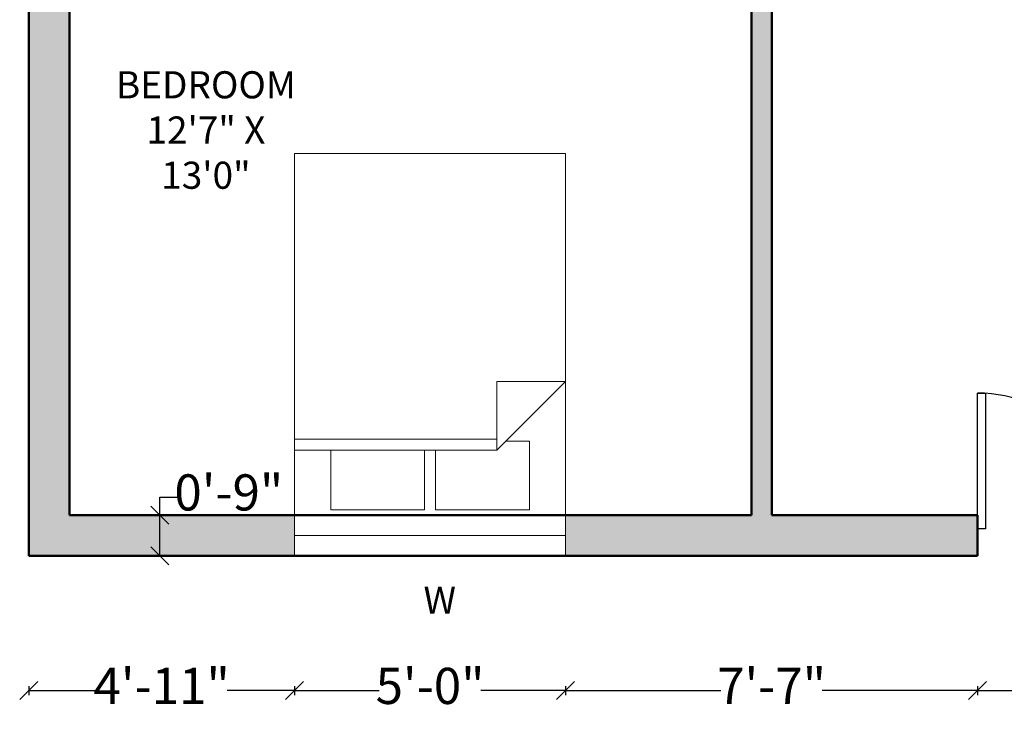
# Model space of a CAD drawing. Units: inches. Extents: x 2395 to 2921, y 528 to 1164.
# Tile 1 of 5: x 2444 to 2662, y 535 to 688. Entities that reach past the tile are written whole.
import ezdxf

# ---------------------------------------------------------------- set-up
doc = ezdxf.new("R2010")
doc.units = ezdxf.units.IN
for name, color, linetype, lineweight in [('A-ANNO-DIMS', 2, 'Continuous', 18), ('A-ANNO-TEXT', 7, 'Continuous', 18), ('A-AREA-IDEN', 7, 'Continuous', 25), ('A-DOOR', 3, 'Continuous', 25), ('A-FURN', 8, 'Continuous', 18), ('A-GLAZ', 4, 'Continuous', 18), ('A-WALL', 162, 'Continuous', 50), ('A-WALL-PATT', 162, 'Continuous', 13)]:
    doc.layers.add(name, color=color, linetype=linetype, lineweight=lineweight)
doc.styles.get("Standard").update_dxf_attribs({"font": 'arial.ttf'})
doc.dimstyles.new('ISO-25', dxfattribs={"dimtxt": 8, "dimasz": 4, "dimexe": 1, "dimexo": 1, "dimtad": 0, "dimtih": 1, "dimtoh": 1, "dimlunit": 3, "dimtxsty": 'Standard', "dimblk": 'OBLIQUE', "dimcen": 2.5, "dimadec": 0, "dimazin": 0, "dimtfac": 1, "dimtmove": 0, "dimatfit": 3, "dimfxl": 1, "dimfxlon": 1, "dimarcsym": 0})

# ---------------------------------------------------------------- blocks, each defined once
blk = doc.blocks.new('*U6')
for p, q in [((0, 0), (0, -6)), ((30, 0), (30, -6))]:
    blk.add_line(p, q)
blk.add_lwpolyline([(0, 0), (0, 30), (1.75, 30), (1.75, 0)], close=True)
blk.add_arc((0, 0), 30, 0, 90)
blk = doc.blocks.new('Bed - Queen')
for p, q in [((0, -80.00003), (0, 0)), ((0, 0), (59.99999, 0)), ((59.99999, 0), (59.99999, -80.00003)), ((7.99999, -1.2), (28.79998, -1.2)), ((7.99999, -14.4), (7.99999, -1.2)), ((28.79998, -1.2), (28.79998, -14.4)), ((31.19999, -1.2), (51.99999, -1.2)), ((31.19999, -14.4), (31.19999, -1.2)), ((51.99999, -1.2), (51.99999, -16.4)), ((0, -14.4), (44.8, -14.4)), ((59.99999, -29.6), (44.8, -14.4)), ((44.8, -14.4), (44.8, -29.6)), ((44.8, -16.8), (0, -16.8)), ((51.99999, -16.4), (46.79936, -16.4)), ((44.8, -29.6), (59.99999, -29.6)), ((59.99999, -80.00003), (0, -80.00003))]:
    blk.add_line(p, q)
blk = doc.blocks.new('_Oblique')
at = {"color": 0, "linetype": 'ByBlock', "lineweight": -2}
blk.add_line((-0.5, -0.5), (0.5, 0.5), dxfattribs=at)
blk = doc.blocks.new('*D42')
at = {"layer": 'A-ANNO-DIMS', "color": 0, "lineweight": -2, "transparency": 16777216}
for p, q in [((2446.2, 541.05), (2446.2, 539.05)), ((2505.03, 541.05), (2505.03, 539.05)), ((2446.2, 540.05), (2461.09, 540.05)), ((2505.03, 540.05), (2490.14, 540.05))]:
    blk.add_line(p, q, dxfattribs=at)
at = {"layer": 'Defpoints', "color": 0, "transparency": 16777216}
for p in [(2446.2, 569.85), (2505.03, 569.85), (2505.03, 540.05)]:
    blk.add_point(p, dxfattribs=at)
at = {"layer": 'A-ANNO-DIMS', "color": 0, "lineweight": -2, "transparency": 16777216, "xscale": 4, "yscale": 4, "zscale": 4, "rotation": 180}
blk.add_blockref('_Oblique', (2446.2, 540.05), dxfattribs=at)
at = {"layer": 'A-ANNO-DIMS', "color": 0, "lineweight": -2, "transparency": 16777216, "xscale": 4, "yscale": 4, "zscale": 4}
blk.add_blockref('_Oblique', (2505.03, 540.05), dxfattribs=at)
at = {"layer": 'A-ANNO-DIMS', "color": 0, "transparency": 16777216, "insert": (2475.62, 540.05), "char_height": 8, "attachment_point": 5}
blk.add_mtext('4\'-11"', dxfattribs=at)
blk = doc.blocks.new('*D43')
at = {"layer": 'A-ANNO-DIMS', "color": 0, "lineweight": -2, "transparency": 16777216}
for p, q in [((2505.03, 541.05), (2505.03, 539.05)), ((2565.03, 541.05), (2565.03, 539.05)), ((2505.03, 540.05), (2523.77, 540.05)), ((2565.03, 540.05), (2546.29, 540.05))]:
    blk.add_line(p, q, dxfattribs=at)
at = {"layer": 'Defpoints', "color": 0, "transparency": 16777216}
for p in [(2505.03, 569.85), (2565.03, 569.85), (2565.03, 540.05)]:
    blk.add_point(p, dxfattribs=at)
at = {"layer": 'A-ANNO-DIMS', "color": 0, "lineweight": -2, "transparency": 16777216, "xscale": 4, "yscale": 4, "zscale": 4, "rotation": 180}
blk.add_blockref('_Oblique', (2505.03, 540.05), dxfattribs=at)
at = {"layer": 'A-ANNO-DIMS', "color": 0, "lineweight": -2, "transparency": 16777216, "xscale": 4, "yscale": 4, "zscale": 4}
blk.add_blockref('_Oblique', (2565.03, 540.05), dxfattribs=at)
at = {"layer": 'A-ANNO-DIMS', "color": 0, "transparency": 16777216, "insert": (2535.03, 540.05), "char_height": 8, "attachment_point": 5}
blk.add_mtext('5\'-0"', dxfattribs=at)
blk = doc.blocks.new('*D44')
at = {"layer": 'A-ANNO-DIMS', "color": 0, "lineweight": -2, "transparency": 16777216}
for p, q in [((2565.03, 541.05), (2565.03, 539.05)), ((2656.2, 541.05), (2656.2, 539.05)), ((2565.03, 540.05), (2599.39, 540.05)), ((2656.2, 540.05), (2621.84, 540.05))]:
    blk.add_line(p, q, dxfattribs=at)
at = {"layer": 'Defpoints', "color": 0, "transparency": 16777216}
for p in [(2565.03, 569.85), (2656.2, 569.85), (2656.2, 540.05)]:
    blk.add_point(p, dxfattribs=at)
at = {"layer": 'A-ANNO-DIMS', "color": 0, "lineweight": -2, "transparency": 16777216, "xscale": 4, "yscale": 4, "zscale": 4, "rotation": 180}
blk.add_blockref('_Oblique', (2565.03, 540.05), dxfattribs=at)
at = {"layer": 'A-ANNO-DIMS', "color": 0, "lineweight": -2, "transparency": 16777216, "xscale": 4, "yscale": 4, "zscale": 4}
blk.add_blockref('_Oblique', (2656.2, 540.05), dxfattribs=at)
at = {"layer": 'A-ANNO-DIMS', "color": 0, "transparency": 16777216, "insert": (2610.62, 540.05), "char_height": 8, "attachment_point": 5}
blk.add_mtext('7\'-7"', dxfattribs=at)
blk = doc.blocks.new('*D45')
at = {"layer": 'A-ANNO-DIMS', "color": 0, "lineweight": -2, "transparency": 16777216}
for p, q in [((2656.2, 541.05), (2656.2, 539.05)), ((2716.2, 541.05), (2716.2, 539.05)), ((2656.2, 540.05), (2674.94, 540.05)), ((2716.2, 540.05), (2697.46, 540.05))]:
    blk.add_line(p, q, dxfattribs=at)
at = {"layer": 'Defpoints', "color": 0, "transparency": 16777216}
for p in [(2656.2, 569.85), (2716.2, 569.85), (2716.2, 540.05)]:
    blk.add_point(p, dxfattribs=at)
at = {"layer": 'A-ANNO-DIMS', "color": 0, "lineweight": -2, "transparency": 16777216, "xscale": 4, "yscale": 4, "zscale": 4, "rotation": 180}
blk.add_blockref('_Oblique', (2656.2, 540.05), dxfattribs=at)
at = {"layer": 'A-ANNO-DIMS', "color": 0, "lineweight": -2, "transparency": 16777216, "xscale": 4, "yscale": 4, "zscale": 4}
blk.add_blockref('_Oblique', (2716.2, 540.05), dxfattribs=at)
at = {"layer": 'A-ANNO-DIMS', "color": 0, "transparency": 16777216, "insert": (2686.2, 540.05), "char_height": 8, "attachment_point": 5}
blk.add_mtext('5\'-0"', dxfattribs=at)
blk = doc.blocks.new('*D50')
at = {"layer": 'A-ANNO-DIMS', "color": 0, "lineweight": -2, "transparency": 16777216}
for p, q in [((2475.23, 578.85), (2475.23, 582.85)), ((2475.23, 582.85), (2479.23, 582.85)), ((2476.23, 578.85), (2474.23, 578.85)), ((2475.23, 569.85), (2475.23, 578.85)), ((2476.23, 569.85), (2474.23, 569.85))]:
    blk.add_line(p, q, dxfattribs=at)
at = {"layer": 'Defpoints', "color": 0, "transparency": 16777216}
for p in [(2475.23, 578.85), (2505.03, 578.85), (2505.03, 569.85)]:
    blk.add_point(p, dxfattribs=at)
at = {"layer": 'A-ANNO-DIMS', "color": 0, "lineweight": -2, "transparency": 16777216, "xscale": 4, "yscale": 4, "zscale": 4}
for p, rotation in [((2475.23, 578.85), 90), ((2475.23, 569.85), 270)]:
    blk.add_blockref('_Oblique', p, dxfattribs=dict(at, rotation=rotation))
at = {"layer": 'A-ANNO-DIMS', "color": 0, "transparency": 16777216, "insert": (2490.49, 582.85), "char_height": 8, "attachment_point": 5}
blk.add_mtext('0\'-9"', dxfattribs=at)
blk = doc.blocks.new('*D51')
at = {"layer": 'A-ANNO-DIMS', "color": 0, "lineweight": -2, "transparency": 16777216}
for p, q in [((2606.2, 1150.65), (2606.2, 1152.65)), ((2606.2, 1151.65), (2610.7, 1151.65)), ((2610.7, 1150.65), (2610.7, 1152.65)), ((2610.7, 1151.65), (2614.7, 1151.65))]:
    blk.add_line(p, q, dxfattribs=at)
at = {"layer": 'Defpoints', "color": 0, "transparency": 16777216}
for p in [(2610.7, 1151.65), (2606.2, 578.85), (2610.7, 578.85)]:
    blk.add_point(p, dxfattribs=at)
at = {"layer": 'A-ANNO-DIMS', "color": 0, "lineweight": -2, "transparency": 16777216, "xscale": 4, "yscale": 4, "zscale": 4, "rotation": 180}
blk.add_blockref('_Oblique', (2606.2, 1151.65), dxfattribs=at)
at = {"layer": 'A-ANNO-DIMS', "color": 0, "lineweight": -2, "transparency": 16777216, "xscale": 4, "yscale": 4, "zscale": 4}
blk.add_blockref('_Oblique', (2610.7, 1151.65), dxfattribs=at)
at = {"layer": 'A-ANNO-DIMS', "color": 0, "transparency": 16777216, "insert": (2635.28, 1151.65), "char_height": 8, "attachment_point": 5}
blk.add_mtext('0\'-4 1/2"', dxfattribs=at)

msp = doc.modelspace()

# ---------------------------------------------------------------- hatches: boundary and pattern name
at = {"layer": 'A-WALL-PATT'}
h = msp.add_hatch(color=256, dxfattribs=at)
h.dxf.hatch_style = 1
h.paths.add_polyline_path([(2627.2, 1121.853), (2446.2, 1121.853), (2446.2, 1054.648), (2455.2, 1054.648), (2455.2, 1112.853), (2606.2, 1112.853), (2606.2, 1022.853), (2610.7, 1022.853), (2610.7, 1112.853), (2627.2, 1112.853)])
h.paths.add_polyline_path([(2685.7, 1121.853), (2648.2, 1121.853), (2648.2, 1112.853), (2664.7, 1112.853), (2664.7, 992.853), (2606.2, 992.853), (2606.2, 962.853), (2610.7, 962.853), (2610.7, 988.353), (2669.2, 988.353), (2669.2, 994.353), (2669.2, 1024.353), (2669.2, 1112.853), (2685.7, 1112.853)])
h.paths.add_polyline_path([(2866.2, 1121.853), (2706.7, 1121.853), (2706.7, 1112.853), (2723.2, 1112.853), (2723.2, 992.853), (2699.2, 992.853), (2699.2, 988.353), (2723.2, 988.353), (2723.2, 962.853), (2727.7, 962.853), (2727.7, 1112.853), (2857.2, 1112.853), (2857.2, 1049.508), (2866.2, 1049.508)])
h.paths.add_polyline_path([(2866.2, 985.129), (2857.2, 985.129), (2857.2, 926.853), (2723.2, 926.853), (2723.2, 922.353), (2729.2, 922.353), (2765.2, 922.353), (2857.2, 922.353), (2857.2, 894.873), (2866.2, 894.873)])
h.paths.add_polyline_path([(2455.2, 997.652), (2446.2, 997.652), (2446.2, 909.181), (2455.2, 908.938), (2455.2, 922.353), (2610.7, 922.353), (2610.7, 926.853), (2455.2, 926.853)])
h.paths.add_polyline_path([(2455.2, 838.353), (2610.7, 838.353), (2610.7, 842.853), (2455.2, 842.853), (2455.2, 856.236), (2446.2, 856.236), (2446.2, 815.427), (2455.2, 815.427)])
h.paths.add_polyline_path([(2455.2, 772.706), (2446.2, 772.706), (2446.2, 569.853), (2505.031, 569.853), (2505.031, 578.853), (2455.2, 578.853), (2455.2, 734.853), (2570.2, 734.853), (2570.2, 739.353), (2568.7, 739.353), (2568.7, 806.353), (2564.2, 806.353), (2564.2, 739.353), (2455.2, 739.353)])
h.paths.add_polyline_path([(2656.2, 578.853), (2610.7, 578.853), (2610.7, 739.353), (2606.2, 739.353), (2606.2, 578.853), (2565.031, 578.853), (2565.031, 569.853), (2656.2, 569.853)])
h.paths.add_polyline_path([(2733.198, 578.853), (2716.2, 578.853), (2716.2, 569.853), (2733.198, 569.853)])
h.paths.add_polyline_path([(2801.188, 578.853), (2764.893, 578.853), (2764.893, 569.853), (2801.188, 569.853)])
h.paths.add_polyline_path([(2866.2, 616.306), (2857.2, 616.306), (2857.2, 578.853), (2836.314, 578.853), (2836.314, 569.853), (2866.2, 569.853)])
h.paths.add_polyline_path([(2866.2, 727.906), (2857.2, 727.906), (2857.2, 670.095), (2866.2, 670.095)])
h.paths.add_polyline_path([(2866.2, 831.149), (2857.2, 831.149), (2857.2, 795.353), (2727.7, 795.353), (2727.7, 886.353), (2723.2, 886.353), (2723.2, 790.853), (2857.2, 790.853), (2857.2, 777.101), (2866.2, 777.101)])

# ---------------------------------------------------------------- linework, layer by layer
at = {"layer": 'A-GLAZ'}
for p, q in [((2505.031, 578.853), (2505.031, 569.853)), ((2565.031, 578.853), (2565.031, 569.853)), ((2565.031, 574.353), (2505.031, 574.353))]:
    msp.add_line(p, q, dxfattribs=at)
at = {"layer": 'A-WALL'}
for p, q in [((2446.2, 1121.853), (2446.2, 569.853)), ((2606.2, 578.853), (2606.2, 739.353)), ((2610.7, 578.853), (2610.7, 739.353)), ((2455.2, 734.853), (2455.2, 578.853)), ((2455.2, 578.853), (2606.2, 578.853)), ((2610.7, 578.853), (2656.2, 578.853)), ((2656.2, 578.853), (2656.2, 569.853)), ((2446.2, 569.853), (2656.2, 569.853))]:
    msp.add_line(p, q, dxfattribs=at)

# ---------------------------------------------------------------- block references
at = {"layer": 'A-DOOR'}
msp.add_blockref('*U6', (2656.2, 575.853), dxfattribs=at)
at = {"layer": 'A-FURN', "xscale": -1, "rotation": 180}
msp.add_blockref('Bed - Queen', (2505.031, 578.853), dxfattribs=at)

# ---------------------------------------------------------------- texts
at = {"layer": 'A-ANNO-TEXT', "insert": (2530.961, 563.042), "char_height": 6, "attachment_point": 1}
msp.add_mtext_dynamic_manual_height_columns('\\pxqc;W', width=12.42697, gutter_width=12.5, heights=[0], dxfattribs=at)
at = {"layer": 'A-AREA-IDEN', "insert": (2465.427, 677.07), "char_height": 6, "attachment_point": 1}
msp.add_mtext_dynamic_manual_height_columns('\\pxqc;BEDROOM\\P12\'7" X 13\'0"', width=39.98375, gutter_width=12.5, heights=[0], dxfattribs=at)

# ---------------------------------------------------------------- dimensions: what is measured, and where the dimension line sits
at = {"layer": 'A-ANNO-DIMS'}
for base, p1, p2, picture, middle in [((2610.7, 1151.653), (2606.2, 578.853), (2610.7, 578.853), '*D51', (2635.278, 1151.653)), ((2505.031, 540.053), (2446.2, 569.853), (2505.031, 569.853), '*D42', (2475.615, 540.053)), ((2565.031, 540.053), (2505.031, 569.853), (2565.031, 569.853), '*D43', (2535.031, 540.053)), ((2656.2, 540.053), (2565.031, 569.853), (2656.2, 569.853), '*D44', (2610.615, 540.053)), ((2716.2, 540.053), (2656.2, 569.853), (2716.2, 569.853), '*D45', (2686.2, 540.053))]:
    dim = msp.add_linear_dim(base=base, p1=p1, p2=p2, dimstyle='ISO-25', override={"dimdec": 1, "dimlfac": 1, "dimrnd": 0, "dimzin": 1, "dimdsep": 46, "dimlunit": 4, "dimfrac": 2}, dxfattribs=at)
    dim.commit()
    dim.dimension.update_dxf_attribs({"geometry": picture, "text_midpoint": middle})
dim = msp.add_linear_dim(base=(2475.231, 578.853), p1=(2505.031, 569.853), p2=(2505.031, 578.853), angle=90, dimstyle='ISO-25', override={"dimdec": 1, "dimlfac": 1, "dimrnd": 0, "dimzin": 1, "dimdsep": 46, "dimlunit": 4, "dimfrac": 2}, dxfattribs=at)
dim.commit()
dim.dimension.update_dxf_attribs({"geometry": '*D50', "text_midpoint": (2490.489, 582.853)})

doc.saveas('drawing.dxf')
